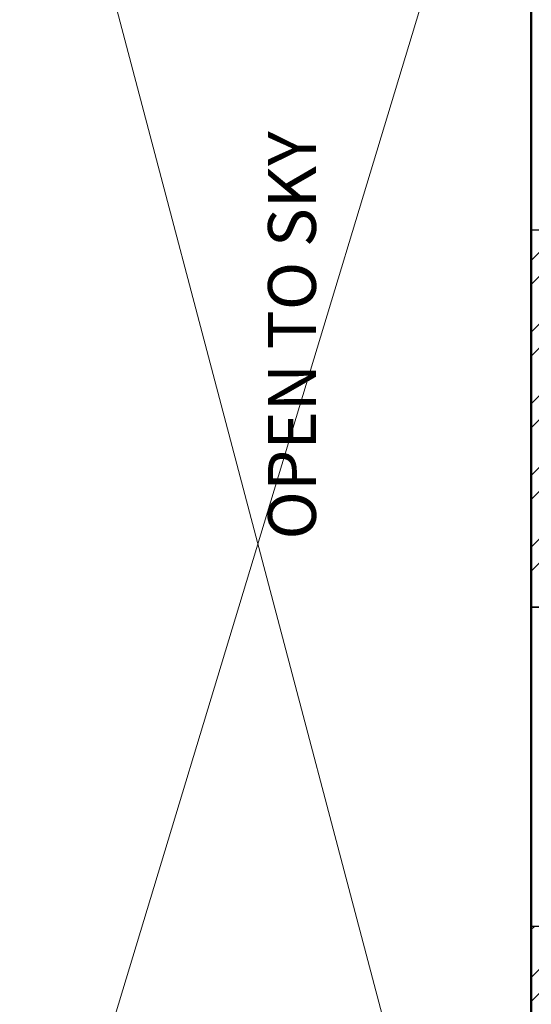
# Model space of a CAD drawing. Units: inches. Extents: x 1901 to 2863, y 888 to 2433.
# Tile 23 of 91: x 2343 to 2439, y 1289 to 1474. Entities that reach past the tile are written whole.
import ezdxf

# ---------------------------------------------------------------- set-up
doc = ezdxf.new("R2010")
doc.units = ezdxf.units.IN
for name, color, linetype, lineweight in [('A-ANNO-SYMB', 8, 'Continuous', 13), ('A-AREA-IDEN', 7, 'Continuous', 18), ('A-GLAZ', 3, 'Continuous', 25), ('A-WALL', 7, 'Continuous', 50), ('A-WALL-PATT', 8, 'Continuous', 13)]:
    doc.layers.add(name, color=color, linetype=linetype, lineweight=lineweight)
doc.styles.get("Standard").update_dxf_attribs({"font": 'arial.ttf'})

# ---------------------------------------------------------------- blocks, each defined once
blk = doc.blocks.new('WIN-60')
for p, q in [((0, 4.5), (0, 0)), ((60, 2.25), (60, 4.5)), ((60, 4.5), (60, 0)), ((0, 0), (0, 2.25)), ((0, 2.25), (60, 2.25))]:
    blk.add_line(p, q)

msp = doc.modelspace()

# ---------------------------------------------------------------- hatches: boundary and pattern name
at = {"layer": 'A-WALL-PATT'}
h = msp.add_hatch(dxfattribs=at)
h.set_pattern_fill('ANSI32', color=256)
h.paths.add_polyline_path([(2192.5, 2274.13), (2141.26, 2274.13), (2141.26, 2269.63), (2192.5, 2269.63)])
h.paths.add_polyline_path([(2259.93, 2274.13), (2216.5, 2274.13), (2216.5, 2269.63), (2255.43, 2269.63), (2255.43, 2214.63), (2250.81, 2214.63), (2250.81, 2210.13), (2259.93, 2210.13), (2259.93, 2215.13), (2271.76, 2215.13), (2271.76, 2217.38), (2271.76, 2219.63), (2259.93, 2219.63)])
h.paths.add_polyline_path([(2171.43, 2269.63), (2166.93, 2269.63), (2166.93, 2219.63), (2121.24, 2219.63), (2121.24, 2215.13), (2166.93, 2215.13), (2166.93, 2083.13), (2161.81, 2083.13), (2161.81, 2078.63), (2171.43, 2078.63), (2177, 2078.63), (2177, 2080.88), (2177, 2083.13), (2171.43, 2083.13), (2171.43, 2210.13), (2230.91, 2210.13), (2230.91, 2212.38), (2230.91, 2214.63), (2171.43, 2214.63)])
h.paths.add_polyline_path([(2117.26, 2274.13), (2089.43, 2274.13), (2089.43, 2219.63), (2081.14, 2219.63), (2081.14, 2215.13), (2089.43, 2215.13), (2098, 2215.13), (2098, 2217.38), (2098, 2219.63), (2093.93, 2219.63), (2093.93, 2269.63), (2117.26, 2269.63), (2117.26, 2271.88)])
h.paths.add_polyline_path([(2343.43, 2219.63), (2329.29, 2219.63), (2329.29, 2215.13), (2338.93, 2215.13), (2338.93, 2184.74), (2343.43, 2184.74)])
h.paths.add_polyline_path([(2338.93, 2083.13), (2329.29, 2083.13), (2208.97, 2083.13), (2208.97, 2078.63), (2338.93, 2078.63)])
h.paths.add_polyline_path([(2343.43, 2136.74), (2338.93, 2136.74), (2338.93, 1872.63), (2343.43, 1872.63)])
h.paths.add_polyline_path([(2343.43, 1863.63), (2397.68, 1863.63), (2397.68, 1821.63), (2384.14, 1821.63), (2384.14, 1812.63), (2418.33, 1812.63), (2418.33, 1817.13), (2418.33, 1821.63), (2406.68, 1821.63), (2406.68, 1863.63), (2459.5, 1863.63), (2459.5, 1821.63), (2447.14, 1821.63), (2447.14, 1812.63), (2459.5, 1812.63), (2468.5, 1812.63), (2468.5, 1872.63), (2394.43, 1872.63), (2334.43, 1872.63), (2334.43, 1812.63), (2343.43, 1812.63), (2353.25, 1812.63), (2353.25, 1821.63), (2343.43, 1821.63)])
h.paths.add_polyline_path([(2510.01, 1872.63), (2468.5, 1872.63), (2468.5, 1868.13), (2510.01, 1868.13)])
h.paths.add_polyline_path([(2514.01, 1817.13), (2468.5, 1817.13), (2468.5, 1812.63), (2482.11, 1812.63), (2482.11, 1800.61), (2486.61, 1800.61), (2486.61, 1812.63), (2514.01, 1812.63)])
h.paths.add_polyline_path([(2299.25, 1814.88), (2299.25, 1817.13), (2295.93, 1817.13), (2295.93, 1854.17), (2293.68, 1854.17), (2291.43, 1854.17), (2291.43, 1817.13), (2266.11, 1817.13), (2266.11, 1812.63), (2299.25, 1812.63)])
h.paths.add_polyline_path([(2218.11, 1817.13), (2206.46, 1817.13), (2171.43, 1817.13), (2171.43, 1949.13), (2190.1, 1949.13), (2190.1, 1953.63), (2163.47, 1953.63), (2163.47, 1949.13), (2166.93, 1949.13), (2166.93, 1817.13), (2114.3, 1817.13), (2114.3, 1812.63), (2218.11, 1812.63)])
h.paths.add_polyline_path([(2029.43, 1970.92), (2024.93, 1970.92), (2024.93, 1912.72), (2029.43, 1912.72)])
h.paths.add_polyline_path([(2132.3, 1953.63), (2113.93, 1953.63), (2113.93, 1975.89), (2111.68, 1975.89), (2109.43, 1975.89), (2109.43, 1953.63), (2029.43, 1953.63), (2029.43, 1949.13), (2132.3, 1949.13)])
h.paths.add_polyline_path([(2029.43, 1853.61), (2029.31, 1853.61), (2029.31, 1853.61), (2029.43, 1853.61), (2029.43, 1864.72), (2024.93, 1864.72), (2024.93, 1812.63), (2066.3, 1812.63), (2066.3, 1814.88), (2066.3, 1817.13), (2029.43, 1817.13)])
h.paths.add_polyline_path([(2122.93, 2010.09), (2120.68, 2010.09), (2118.43, 2010.09), (2118.43, 2006.13), (2029.43, 2006.13), (2029.43, 2001.63), (2109.43, 2001.63), (2109.43, 1998.04), (2113.93, 1998.04), (2113.93, 2001.63), (2122.93, 2001.63)])
h.paths.add_polyline_path([(2029.43, 2031.38), (2024.93, 2031.38), (2024.93, 1994.92), (2027.18, 1994.92), (2029.43, 1994.92)])
h.paths.add_polyline_path([(2029.43, 2136.74), (2024.93, 2136.74), (2024.93, 2067.38), (2027.18, 2067.38), (2029.43, 2067.38)])
h.paths.add_polyline_path([(2125.62, 2083.13), (2029.43, 2083.13), (2029.43, 2078.63), (2118.43, 2078.63), (2118.43, 2030.71), (2122.93, 2030.71), (2122.93, 2078.63), (2125.62, 2078.63)])
h.paths.add_polyline_path([(2029.43, 2215.13), (2040.47, 2215.13), (2040.47, 2217.38), (2040.47, 2219.63), (2024.93, 2219.63), (2024.93, 2184.74), (2029.43, 2184.74), (2029.43, 2187.78)])
h.paths.add_polyline_path([(2686.43, 2274.13), (2659.28, 2274.13), (2659.28, 2269.63), (2681.93, 2269.63), (2681.93, 2219.63), (2676.82, 2219.63), (2676.82, 2215.13), (2681.93, 2215.13), (2697.01, 2215.13), (2697.01, 2217.38), (2697.01, 2219.63), (2686.43, 2219.63)])
h.paths.add_polyline_path([(2609.93, 2269.63), (2635.28, 2269.63), (2635.28, 2274.13), (2571.43, 2274.13), (2571.43, 2269.63), (2605.43, 2269.63), (2605.43, 2214.63), (2549.1, 2214.63), (2549.1, 2210.13), (2605.43, 2210.13), (2605.43, 2083.13), (2601.01, 2083.13), (2601.01, 2080.88), (2601.01, 2078.63), (2609.93, 2078.63), (2616.16, 2078.63), (2616.16, 2080.88), (2616.16, 2083.13), (2609.93, 2083.13), (2609.93, 2215.13), (2651.46, 2215.13), (2651.46, 2217.38), (2651.46, 2219.63), (2609.93, 2219.63)])
h.paths.add_polyline_path([(2521.43, 2269.63), (2547.43, 2269.63), (2547.43, 2271.88), (2547.43, 2274.13), (2516.93, 2274.13), (2516.93, 2219.63), (2506.41, 2219.63), (2506.41, 2215.13), (2516.93, 2215.13), (2516.93, 2210.13), (2525.4, 2210.13), (2525.4, 2212.38), (2525.4, 2214.63), (2521.43, 2214.63)])
h.paths.add_polyline_path([(2456.01, 2219.63), (2439.43, 2219.63), (2439.43, 2187.89), (2443.93, 2187.89), (2443.93, 2215.13), (2456.01, 2215.13)])
h.paths.add_polyline_path([(2752.93, 2219.63), (2739.48, 2219.63), (2739.48, 2215.13), (2748.43, 2215.13), (2748.43, 2187.89), (2752.93, 2187.89)])
h.paths.add_polyline_path([(2752.93, 2139.89), (2748.43, 2139.89), (2748.43, 2083.13), (2648.42, 2083.13), (2648.42, 2078.63), (2654.93, 2078.63), (2654.93, 2039.44), (2659.43, 2039.44), (2659.43, 2078.63), (2748.43, 2078.63), (2748.43, 2063.43), (2752.93, 2063.43)])
h.paths.add_polyline_path([(2752.93, 2010.63), (2659.43, 2010.63), (2659.43, 2015.65), (2654.93, 2015.65), (2654.93, 2010.63), (2605.43, 2010.63), (2605.43, 1920.97), (2609.93, 1920.97), (2609.93, 2006.13), (2748.43, 2006.13), (2748.43, 1982.47), (2752.93, 1982.47)])
h.paths.add_polyline_path([(2752.93, 2027.43), (2748.43, 2027.43), (2748.43, 2010.63), (2752.93, 2010.63)])
h.paths.add_polyline_path([(2748.43, 1886.13), (2609.93, 1886.13), (2609.93, 1889.72), (2605.43, 1889.72), (2605.43, 1861.26), (2609.93, 1861.26), (2609.93, 1881.63), (2748.43, 1881.63)])
h.paths.add_polyline_path([(2456.86, 2228.83), (2498.4, 2228.83), (2498.4, 2247.49), (2456.86, 2247.49)], flags=9)
h.paths.add_polyline_path([(2038.6, 2237.42), (2080.17, 2237.42), (2080.17, 2256.08), (2038.6, 2256.08)], flags=9)
h.paths.add_polyline_path([(2292.01, 1062.39), (2539.93, 1062.39), (2539.93, 1099.49), (2292.01, 1099.49)], flags=9)
h.paths.add_polyline_path([(2424.91, 1832.25), (2448.51, 1832.25), (2448.51, 1846.68), (2424.91, 1846.68)], flags=25)
h.paths.add_polyline_path([(2359.08, 1832.25), (2382.68, 1832.25), (2382.68, 1846.68), (2359.08, 1846.68)], flags=25)
h.paths.add_polyline_path([(2352.9, 1684.8), (2367.54, 1684.8), (2367.54, 1697.17), (2352.9, 1697.17)], flags=9)
h.paths.add_polyline_path([(2079.29, 1755.83), (2169.02, 1755.83), (2169.02, 1774.37), (2079.29, 1774.37)], flags=9)
h.paths.add_polyline_path([(2404.09, 1373.86), (2404.09, 1463.59), (2385.54, 1463.59), (2385.54, 1373.86)], flags=9)
h.paths.add_polyline_path([(2268.09, 2236.37), (2309.64, 2236.37), (2309.64, 2255.03), (2268.09, 2255.03)], flags=9)
h.paths.add_polyline_path([(2575.96, 1700.95), (2665.7, 1700.95), (2665.7, 1719.5), (2575.96, 1719.5)], flags=9)
h.paths.add_polyline_path([(2302.96, 1878.47), (2329.52, 1878.47), (2329.52, 1888.78), (2302.96, 1888.78)], flags=9)
h.paths.add_polyline_path([(2097.42, 2240.58), (2126.57, 2240.58), (2126.57, 2259.23), (2097.42, 2259.23)], flags=9)
h.paths.add_polyline_path([(2208.72, 2246.12), (2237.88, 2246.12), (2237.88, 2264.78), (2208.72, 2264.78)], flags=9)
h.paths.add_polyline_path([(2038.15, 1925.96), (2076.99, 1925.96), (2076.99, 1944.62), (2038.15, 1944.62)], flags=9)
h.paths.add_polyline_path([(2239.14, 1926.67), (2288.46, 1926.67), (2288.46, 1945.33), (2239.14, 1945.33)], flags=9)
h.paths.add_polyline_path([(2175.43, 2007.33), (2212.36, 2007.33), (2212.36, 2025.99), (2175.43, 2025.99)], flags=9)
h.paths.add_polyline_path([(2225.03, 2091.79), (2263.87, 2091.79), (2263.87, 2110.45), (2225.03, 2110.45)], flags=9)
h.paths.add_polyline_path([(2035.4, 2098.48), (2074.24, 2098.48), (2074.24, 2117.14), (2035.4, 2117.14)], flags=9)
h.paths.add_polyline_path([(2050.1, 2029.21), (2083.26, 2029.21), (2083.26, 2047.87), (2050.1, 2047.87)], flags=9)
h.paths.add_polyline_path([(2069.68, 1956.72), (2098.83, 1956.72), (2098.83, 1975.38), (2069.68, 1975.38)], flags=25)
h.paths.add_polyline_path([(2328.62, 1753.34), (2361.66, 1753.34), (2361.66, 1771.99), (2328.62, 1771.99)], flags=9)
h.paths.add_polyline_path([(2395.16, 2060.89), (2395.16, 2140.65), (2378.68, 2140.65), (2378.68, 2060.89)], flags=9)
h.paths.add_polyline_path([(2463.73, 2059.02), (2492.89, 2059.02), (2492.89, 2077.68), (2463.73, 2077.68)], flags=9)
h.paths.add_polyline_path([(2458.03, 2181.54), (2496.87, 2181.54), (2496.87, 2200.19), (2458.03, 2200.19)], flags=9)
h.paths.add_polyline_path([(2527.58, 2243.07), (2556.73, 2243.07), (2556.73, 2261.73), (2527.58, 2261.73)], flags=9)
h.paths.add_polyline_path([(2694.46, 2232.77), (2736.03, 2232.77), (2736.03, 2251.42), (2694.46, 2251.42)], flags=9)
h.paths.add_polyline_path([(2637.82, 2249.22), (2666.98, 2249.22), (2666.98, 2267.88), (2637.82, 2267.88)], flags=9)
h.paths.add_polyline_path([(2623.69, 2183.54), (2662.53, 2183.54), (2662.53, 2202.2), (2623.69, 2202.2)], flags=9)
h.paths.add_polyline_path([(2691.97, 2021.5), (2725.12, 2021.5), (2725.12, 2040.16), (2691.97, 2040.16)], flags=9)
h.paths.add_polyline_path([(2621.04, 1975.91), (2662.34, 1975.91), (2662.34, 1994.57), (2621.04, 1994.57)], flags=25)
h.paths.add_polyline_path([(2479.03, 1927.62), (2519.84, 1927.62), (2519.84, 1946.28), (2479.03, 1946.28)], flags=9)
h.paths.add_polyline_path([(2670.94, 1849.08), (2716.01, 1849.08), (2716.01, 1867.73), (2670.94, 1867.73)], flags=9)
h.paths.add_polyline_path([(2523.61, 1782.96), (2550.17, 1782.96), (2550.17, 1793.26), (2523.61, 1793.26)], flags=9)
h.paths.add_polyline_path([(2450.84, 1207.33), (2492.39, 1207.33), (2492.39, 1225.99), (2450.84, 1225.99)], flags=9)
h.paths.add_polyline_path([(2527.75, 1203.84), (2556.91, 1203.84), (2556.91, 1222.5), (2527.75, 1222.5)], flags=9)
h.paths.add_polyline_path([(2639.11, 1207.2), (2668.27, 1207.2), (2668.27, 1225.86), (2639.11, 1225.86)], flags=9)
h.paths.add_polyline_path([(2692.59, 1218.97), (2734.17, 1218.97), (2734.17, 1237.62), (2692.59, 1237.62)], flags=9)
h.paths.add_polyline_path([(2669.27, 1366.33), (2708.11, 1366.33), (2708.11, 1384.99), (2669.27, 1384.99)], flags=9)
h.paths.add_polyline_path([(2463.31, 1358.03), (2502.15, 1358.03), (2502.15, 1376.69), (2463.31, 1376.69)], flags=9)
h.paths.add_polyline_path([(2494.72, 1449.96), (2531.65, 1449.96), (2531.65, 1468.62), (2494.72, 1468.62)], flags=9)
h.paths.add_polyline_path([(2675.57, 1422.16), (2708.72, 1422.16), (2708.72, 1440.81), (2675.57, 1440.81)], flags=9)
h.paths.add_polyline_path([(2685.63, 1493.89), (2714.79, 1493.89), (2714.79, 1512.55), (2685.63, 1512.55)], flags=9)
h.paths.add_polyline_path([(2686.8, 1529.91), (2725.65, 1529.91), (2725.65, 1548.57), (2686.8, 1548.57)], flags=9)
h.paths.add_polyline_path([(2503.65, 1537.99), (2552.97, 1537.99), (2552.97, 1556.65), (2503.65, 1556.65)], flags=9)
h.paths.add_polyline_path([(2291.71, 1643.5), (2318.28, 1643.5), (2318.28, 1653.81), (2291.71, 1653.81)], flags=9)
h.paths.add_polyline_path([(2450.63, 1610.52), (2477.19, 1610.52), (2477.19, 1620.82), (2450.63, 1620.82)], flags=9)
h.paths.add_polyline_path([(2359.99, 1551.81), (2422.25, 1551.81), (2422.25, 1562.12), (2359.99, 1562.12)], flags=9)
h.paths.add_polyline_path([(2280.11, 1249.01), (2321.65, 1249.01), (2321.65, 1267.66), (2280.11, 1267.66)], flags=9)
h.paths.add_polyline_path([(2164.06, 1274.23), (2193.22, 1274.23), (2193.22, 1292.89), (2164.06, 1292.89)], flags=9)
h.paths.add_polyline_path([(2118.21, 1277.69), (2151.25, 1277.69), (2151.25, 1296.35), (2118.21, 1296.35)], flags=9)
h.paths.add_polyline_path([(2031.95, 1268.53), (2073.52, 1268.53), (2073.52, 1287.19), (2031.95, 1287.19)], flags=9)
h.paths.add_polyline_path([(2050.2, 1409.08), (2089.04, 1409.08), (2089.04, 1427.74), (2050.2, 1427.74)], flags=9)
h.paths.add_polyline_path([(2243.74, 1421.03), (2282.58, 1421.03), (2282.58, 1439.69), (2243.74, 1439.69)], flags=9)
h.paths.add_polyline_path([(2190.75, 1509.77), (2231.56, 1509.77), (2231.56, 1528.43), (2190.75, 1528.43)], flags=9)
h.paths.add_polyline_path([(2058.39, 1475.42), (2091.55, 1475.42), (2091.55, 1494.07), (2058.39, 1494.07)], flags=9)
h.paths.add_polyline_path([(2062.45, 1553.09), (2091.6, 1553.09), (2091.6, 1571.75), (2062.45, 1571.75)], flags=9)
h.paths.add_polyline_path([(2219.52, 1590.37), (2266.15, 1590.37), (2266.15, 1609.02), (2219.52, 1609.02)], flags=9)
h.paths.add_polyline_path([(2041.07, 1584.19), (2079.91, 1584.19), (2079.91, 1602.85), (2041.07, 1602.85)], flags=9)
h = msp.add_hatch(dxfattribs=at)
h.set_pattern_fill('ANSI32', color=256)
h.paths.add_polyline_path([(2443.93, 2139.89), (2439.43, 2139.89), (2439.43, 2069.35), (2441.68, 2069.35), (2443.93, 2069.35), (2443.93, 2078.63), (2521.93, 2078.63), (2521.93, 2075.07), (2524.18, 2075.07), (2526.43, 2075.07), (2526.43, 2078.63), (2571.75, 2078.63), (2571.75, 2080.88), (2571.75, 2083.13), (2443.93, 2083.13)])
h.paths.add_polyline_path([(2526.43, 2054.63), (2524.18, 2054.63), (2521.93, 2054.63), (2521.93, 2030.63), (2443.93, 2030.63), (2443.93, 2045.35), (2439.43, 2045.35), (2439.43, 1983.87), (2443.93, 1983.87), (2443.93, 2026.13), (2521.93, 2026.13), (2526.43, 2026.13)])
h.paths.add_polyline_path([(2443.93, 1923.87), (2439.43, 1923.87), (2439.43, 1872.63), (2443.93, 1872.63)])
h.paths.add_polyline_path([(2636.23, 1766.13), (2609.93, 1766.13), (2609.93, 1779.79), (2605.43, 1779.79), (2605.43, 1766.13), (2486.61, 1766.13), (2486.61, 1770.67), (2482.11, 1770.67), (2482.11, 1766.13), (2482.11, 1761.63), (2636.23, 1761.63), (2636.23, 1763.88)])
h.paths.add_polyline_path([(2519.54, 1663.38), (2519.54, 1665.63), (2494.93, 1665.63), (2481.83, 1665.63), (2481.83, 1663.38), (2481.83, 1661.13), (2490.43, 1661.13), (2490.43, 1640.16), (2494.93, 1640.16), (2494.93, 1661.13), (2519.54, 1661.13)])
h.paths.add_polyline_path([(2443.93, 1712.13), (2443.93, 1716.63), (2414.46, 1716.63), (2414.46, 1712.13), (2439.43, 1712.13), (2439.43, 1545.51), (2443.93, 1545.51), (2443.93, 1661.13), (2448.47, 1661.13), (2448.47, 1665.63), (2443.93, 1665.63)])
h.paths.add_polyline_path([(2343.43, 1712.13), (2365.52, 1712.13), (2365.52, 1714.38), (2365.52, 1716.63), (2333.87, 1716.63), (2333.87, 1714.38), (2333.87, 1712.13), (2338.93, 1712.13), (2338.93, 1575.63), (2338.93, 1545.51), (2343.43, 1545.51), (2343.43, 1547.51), (2343.43, 1580.13)])
h.paths.add_polyline_path([(2752.93, 1665.63), (2579.54, 1665.63), (2579.54, 1661.13), (2615.93, 1661.13), (2615.93, 1529.13), (2598.93, 1529.13), (2598.93, 1524.63), (2623.13, 1524.63), (2623.13, 1526.88), (2623.13, 1529.13), (2620.43, 1529.13), (2620.43, 1661.13), (2748.43, 1661.13), (2748.43, 1633.5), (2752.93, 1633.5)])
h.paths.add_polyline_path([(2752.93, 1419.93), (2748.43, 1419.93), (2748.43, 1400.13), (2659.43, 1400.13), (2659.43, 1444.33), (2657.18, 1444.33), (2654.93, 1444.33), (2654.93, 1400.13), (2643.65, 1400.13), (2643.65, 1395.63), (2748.43, 1395.63), (2748.43, 1364.04), (2752.93, 1364.04)])
h.paths.add_polyline_path([(2752.93, 1492.88), (2748.43, 1492.88), (2748.43, 1476.63), (2667.43, 1476.63), (2667.43, 1479.71), (2665.18, 1479.71), (2662.93, 1479.71), (2662.93, 1476.63), (2654.93, 1476.63), (2654.93, 1469.54), (2659.43, 1469.54), (2659.43, 1472.13), (2748.43, 1472.13), (2748.43, 1455.93), (2752.93, 1455.93)])
h.paths.add_polyline_path([(2752.93, 1304.04), (2748.43, 1304.04), (2748.43, 1263.63), (2738.66, 1263.63), (2738.66, 1259.13), (2752.93, 1259.13)])
h.paths.add_polyline_path([(2685.93, 1259.13), (2695.49, 1259.13), (2695.49, 1261.38), (2695.49, 1263.63), (2677.84, 1263.63), (2677.84, 1261.38), (2677.84, 1259.13), (2681.43, 1259.13), (2681.43, 1203.63), (2653.28, 1203.63), (2653.28, 1199.13), (2685.93, 1199.13), (2685.93, 1203.63)])
h.paths.add_polyline_path([(2609.43, 1395.63), (2611.85, 1395.63), (2611.85, 1400.13), (2598.89, 1400.13), (2598.89, 1397.88), (2598.89, 1395.63), (2604.93, 1395.63), (2604.93, 1268.13), (2554.73, 1268.13), (2554.73, 1265.88), (2554.73, 1263.63), (2604.93, 1263.63), (2604.93, 1203.63), (2571.31, 1203.63), (2571.31, 1199.13), (2604.93, 1199.13), (2629.28, 1199.13), (2629.28, 1201.38), (2629.28, 1203.63), (2609.43, 1203.63), (2609.43, 1258.63), (2609.43, 1259.13), (2654.8, 1259.13), (2654.8, 1263.63), (2609.43, 1263.63)])
h.paths.add_polyline_path([(2443.93, 1304.04), (2439.43, 1304.04), (2439.43, 1259.13), (2443.93, 1259.13), (2456.16, 1259.13), (2456.16, 1261.38), (2456.16, 1263.63), (2443.93, 1263.63)])
h.paths.add_polyline_path([(2525.43, 1263.63), (2531.78, 1263.63), (2531.78, 1268.13), (2520.93, 1268.13), (2520.93, 1263.63), (2511.41, 1263.63), (2511.41, 1259.13), (2520.93, 1259.13), (2520.93, 1199.13), (2547.31, 1199.13), (2547.31, 1201.38), (2547.31, 1203.63), (2525.43, 1203.63)])
h.paths.add_polyline_path([(2443.93, 1434.84), (2439.43, 1434.84), (2439.43, 1364.04), (2441.68, 1364.04), (2443.93, 1364.04)])
h.paths.add_polyline_path([(2567.13, 1400.13), (2443.93, 1400.13), (2443.93, 1395.63), (2567.13, 1395.63)])
h.paths.add_polyline_path([(2443.93, 1545.51), (2439.43, 1545.51), (2439.43, 1494.84), (2443.93, 1494.84)])
h.paths.add_polyline_path([(2494.93, 1553.35), (2492.68, 1553.35), (2490.43, 1553.35), (2490.43, 1524.63), (2494.93, 1524.63), (2525.94, 1524.63), (2525.94, 1526.88), (2525.94, 1529.13), (2494.93, 1529.13)])
h.paths.add_polyline_path([(2752.93, 1573.5), (2748.43, 1573.5), (2748.43, 1529.13), (2657.76, 1529.13), (2657.76, 1524.63), (2662.93, 1524.63), (2662.93, 1498.63), (2667.43, 1498.63), (2667.43, 1524.63), (2748.43, 1524.63), (2748.43, 1516.88), (2752.93, 1516.88)])
h.paths.add_polyline_path([(2038.6, 2237.42), (2080.17, 2237.42), (2080.17, 2256.08), (2038.6, 2256.08)], flags=9)
h.paths.add_polyline_path([(2292.01, 1062.39), (2539.93, 1062.39), (2539.93, 1099.49), (2292.01, 1099.49)], flags=9)
h.paths.add_polyline_path([(2424.91, 1832.25), (2448.51, 1832.25), (2448.51, 1846.68), (2424.91, 1846.68)], flags=9)
h.paths.add_polyline_path([(2359.08, 1832.25), (2382.68, 1832.25), (2382.68, 1846.68), (2359.08, 1846.68)], flags=9)
h.paths.add_polyline_path([(2352.9, 1684.8), (2367.54, 1684.8), (2367.54, 1697.17), (2352.9, 1697.17)], flags=9)
h.paths.add_polyline_path([(2079.29, 1755.83), (2169.02, 1755.83), (2169.02, 1774.37), (2079.29, 1774.37)], flags=9)
h.paths.add_polyline_path([(2404.09, 1373.86), (2404.09, 1463.59), (2385.54, 1463.59), (2385.54, 1373.86)], flags=9)
h.paths.add_polyline_path([(2268.09, 2236.37), (2309.64, 2236.37), (2309.64, 2255.03), (2268.09, 2255.03)], flags=9)
h.paths.add_polyline_path([(2575.96, 1700.95), (2665.7, 1700.95), (2665.7, 1719.5), (2575.96, 1719.5)], flags=9)
h.paths.add_polyline_path([(2302.96, 1878.47), (2329.52, 1878.47), (2329.52, 1888.78), (2302.96, 1888.78)], flags=9)
h.paths.add_polyline_path([(2097.42, 2240.58), (2126.57, 2240.58), (2126.57, 2259.23), (2097.42, 2259.23)], flags=9)
h.paths.add_polyline_path([(2208.72, 2246.12), (2237.88, 2246.12), (2237.88, 2264.78), (2208.72, 2264.78)], flags=9)
h.paths.add_polyline_path([(2038.15, 1925.96), (2076.99, 1925.96), (2076.99, 1944.62), (2038.15, 1944.62)], flags=9)
h.paths.add_polyline_path([(2239.14, 1926.67), (2288.46, 1926.67), (2288.46, 1945.33), (2239.14, 1945.33)], flags=9)
h.paths.add_polyline_path([(2175.43, 2007.33), (2212.36, 2007.33), (2212.36, 2025.99), (2175.43, 2025.99)], flags=9)
h.paths.add_polyline_path([(2225.03, 2091.79), (2263.87, 2091.79), (2263.87, 2110.45), (2225.03, 2110.45)], flags=9)
h.paths.add_polyline_path([(2035.4, 2098.48), (2074.24, 2098.48), (2074.24, 2117.14), (2035.4, 2117.14)], flags=9)
h.paths.add_polyline_path([(2050.1, 2029.21), (2083.26, 2029.21), (2083.26, 2047.87), (2050.1, 2047.87)], flags=9)
h.paths.add_polyline_path([(2069.68, 1956.72), (2098.83, 1956.72), (2098.83, 1975.38), (2069.68, 1975.38)], flags=9)
h.paths.add_polyline_path([(2328.62, 1753.34), (2361.66, 1753.34), (2361.66, 1771.99), (2328.62, 1771.99)], flags=9)
h.paths.add_polyline_path([(2395.16, 2060.89), (2395.16, 2140.65), (2378.68, 2140.65), (2378.68, 2060.89)], flags=9)
h.paths.add_polyline_path([(2463.73, 2059.02), (2492.89, 2059.02), (2492.89, 2077.68), (2463.73, 2077.68)], flags=9)
h.paths.add_polyline_path([(2458.03, 2181.54), (2496.87, 2181.54), (2496.87, 2200.19), (2458.03, 2200.19)], flags=9)
h.paths.add_polyline_path([(2456.86, 2228.83), (2498.4, 2228.83), (2498.4, 2247.49), (2456.86, 2247.49)], flags=9)
h.paths.add_polyline_path([(2527.58, 2243.07), (2556.73, 2243.07), (2556.73, 2261.73), (2527.58, 2261.73)], flags=9)
h.paths.add_polyline_path([(2694.46, 2232.77), (2736.03, 2232.77), (2736.03, 2251.42), (2694.46, 2251.42)], flags=9)
h.paths.add_polyline_path([(2637.82, 2249.22), (2666.98, 2249.22), (2666.98, 2267.88), (2637.82, 2267.88)], flags=9)
h.paths.add_polyline_path([(2623.69, 2183.54), (2662.53, 2183.54), (2662.53, 2202.2), (2623.69, 2202.2)], flags=9)
h.paths.add_polyline_path([(2691.97, 2021.5), (2725.12, 2021.5), (2725.12, 2040.16), (2691.97, 2040.16)], flags=9)
h.paths.add_polyline_path([(2621.04, 1975.91), (2662.34, 1975.91), (2662.34, 1994.57), (2621.04, 1994.57)], flags=9)
h.paths.add_polyline_path([(2479.03, 1927.62), (2519.84, 1927.62), (2519.84, 1946.28), (2479.03, 1946.28)], flags=9)
h.paths.add_polyline_path([(2670.94, 1849.08), (2716.01, 1849.08), (2716.01, 1867.73), (2670.94, 1867.73)], flags=9)
h.paths.add_polyline_path([(2523.61, 1782.96), (2550.17, 1782.96), (2550.17, 1793.26), (2523.61, 1793.26)], flags=9)
h.paths.add_polyline_path([(2450.84, 1207.33), (2492.39, 1207.33), (2492.39, 1225.99), (2450.84, 1225.99)], flags=9)
h.paths.add_polyline_path([(2527.75, 1203.84), (2556.91, 1203.84), (2556.91, 1222.5), (2527.75, 1222.5)], flags=9)
h.paths.add_polyline_path([(2639.11, 1207.2), (2668.27, 1207.2), (2668.27, 1225.86), (2639.11, 1225.86)], flags=9)
h.paths.add_polyline_path([(2692.59, 1218.97), (2734.17, 1218.97), (2734.17, 1237.62), (2692.59, 1237.62)], flags=9)
h.paths.add_polyline_path([(2669.27, 1366.33), (2708.11, 1366.33), (2708.11, 1384.99), (2669.27, 1384.99)], flags=25)
h.paths.add_polyline_path([(2463.31, 1358.03), (2502.15, 1358.03), (2502.15, 1376.69), (2463.31, 1376.69)], flags=9)
h.paths.add_polyline_path([(2494.72, 1449.96), (2531.65, 1449.96), (2531.65, 1468.62), (2494.72, 1468.62)], flags=9)
h.paths.add_polyline_path([(2675.57, 1422.16), (2708.72, 1422.16), (2708.72, 1440.81), (2675.57, 1440.81)], flags=25)
h.paths.add_polyline_path([(2685.63, 1493.89), (2714.79, 1493.89), (2714.79, 1512.55), (2685.63, 1512.55)], flags=9)
h.paths.add_polyline_path([(2686.8, 1529.91), (2725.65, 1529.91), (2725.65, 1548.57), (2686.8, 1548.57)], flags=25)
h.paths.add_polyline_path([(2503.65, 1537.99), (2552.97, 1537.99), (2552.97, 1556.65), (2503.65, 1556.65)], flags=9)
h.paths.add_polyline_path([(2291.71, 1643.5), (2318.28, 1643.5), (2318.28, 1653.81), (2291.71, 1653.81)], flags=9)
h.paths.add_polyline_path([(2450.63, 1610.52), (2477.19, 1610.52), (2477.19, 1620.82), (2450.63, 1620.82)], flags=9)
h.paths.add_polyline_path([(2359.99, 1551.81), (2422.25, 1551.81), (2422.25, 1562.12), (2359.99, 1562.12)], flags=9)
h.paths.add_polyline_path([(2280.11, 1249.01), (2321.65, 1249.01), (2321.65, 1267.66), (2280.11, 1267.66)], flags=9)
h.paths.add_polyline_path([(2164.06, 1274.23), (2193.22, 1274.23), (2193.22, 1292.89), (2164.06, 1292.89)], flags=9)
h.paths.add_polyline_path([(2118.21, 1277.69), (2151.25, 1277.69), (2151.25, 1296.35), (2118.21, 1296.35)], flags=9)
h.paths.add_polyline_path([(2031.95, 1268.53), (2073.52, 1268.53), (2073.52, 1287.19), (2031.95, 1287.19)], flags=9)
h.paths.add_polyline_path([(2050.2, 1409.08), (2089.04, 1409.08), (2089.04, 1427.74), (2050.2, 1427.74)], flags=9)
h.paths.add_polyline_path([(2243.74, 1421.03), (2282.58, 1421.03), (2282.58, 1439.69), (2243.74, 1439.69)], flags=9)
h.paths.add_polyline_path([(2190.75, 1509.77), (2231.56, 1509.77), (2231.56, 1528.43), (2190.75, 1528.43)], flags=9)
h.paths.add_polyline_path([(2058.39, 1475.42), (2091.55, 1475.42), (2091.55, 1494.07), (2058.39, 1494.07)], flags=9)
h.paths.add_polyline_path([(2062.45, 1553.09), (2091.6, 1553.09), (2091.6, 1571.75), (2062.45, 1571.75)], flags=9)
h.paths.add_polyline_path([(2219.52, 1590.37), (2266.15, 1590.37), (2266.15, 1609.02), (2219.52, 1609.02)], flags=9)
h.paths.add_polyline_path([(2041.07, 1584.19), (2079.91, 1584.19), (2079.91, 1602.85), (2041.07, 1602.85)], flags=9)

# ---------------------------------------------------------------- linework, layer by layer
at = {"layer": 'A-ANNO-SYMB'}
for p, q in [((2343.43, 1228.13), (2439.43, 1545.51)), ((2343.43, 1545.51), (2439.43, 1181.13))]:
    msp.add_line(p, q, dxfattribs=at)
at = {"layer": 'A-WALL'}
msp.add_line((2439.43, 1259.13), (2439.43, 1712.13), dxfattribs=at)

# ---------------------------------------------------------------- block references
at = {"layer": 'A-GLAZ', "rotation": 270.0000000000005}
for p in [(2439.43, 1494.84), (2439.43, 1364.04)]:
    msp.add_blockref('WIN-60', p, dxfattribs=at)

# ---------------------------------------------------------------- texts
at = {"layer": 'A-AREA-IDEN', "insert": (2390.02, 1376.71), "char_height": 9, "attachment_point": 1, "rotation": 90}
msp.add_mtext_dynamic_manual_height_columns('OPEN TO SKY', width=303.7811, gutter_width=12.5, heights=[0], dxfattribs=at)

doc.saveas('drawing.dxf')
